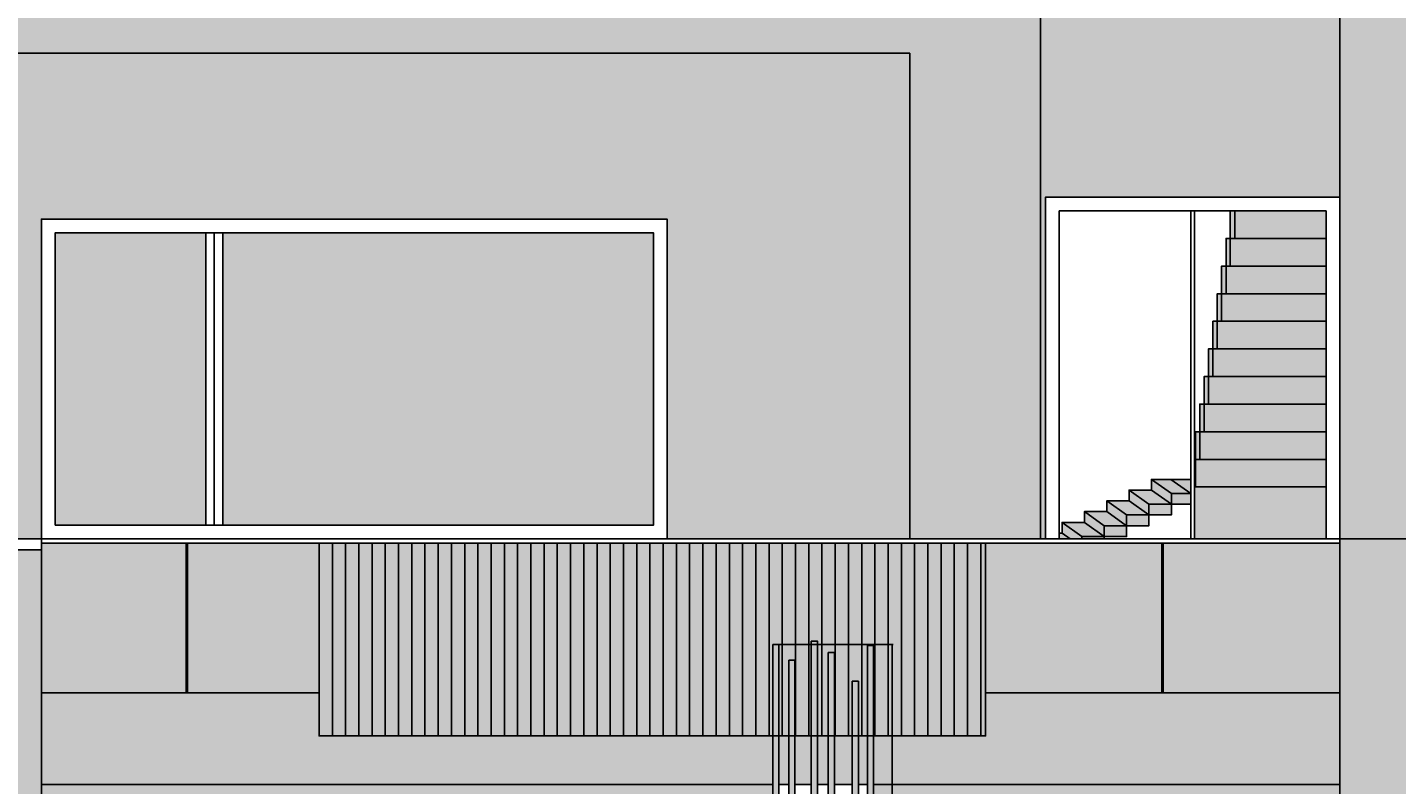
# Model space of a CAD drawing. Units: feet. Extents: x 2193 to 3502, y 890 to 1601.
# Tile 6 of 17: x 2466 to 2710, y 1225 to 1360. Entities that reach past the tile are written whole.
import ezdxf

# ---------------------------------------------------------------- set-up
doc = ezdxf.new("R2010")
doc.units = ezdxf.units.FT
for name, color, linetype, lineweight in [('A-ANNO-DIMS', 2, 'Continuous', 18), ('A-ELEV', 7, 'Continuous', 25), ('A-ELEV-PATT', 8, 'Continuous', 13)]:
    doc.layers.add(name, color=color, linetype=linetype, lineweight=lineweight)
doc.styles.get("Standard").update_dxf_attribs({"font": 'arial.ttf'})
doc.dimstyles.get("Standard").update_dxf_attribs({"dimtxt": 0.18, "dimasz": 0.18, "dimexe": 0.18, "dimexo": 0.0625, "dimgap": 0.09, "dimtad": 0, "dimtih": 1, "dimtoh": 1, "dimdec": 0, "dimzin": 0, "dimdsep": 46, "dimlunit": 3, "dimtxsty": 'Standard', "dimcen": 0.09, "dimadec": 0, "dimazin": 0, "dimtfac": 1, "dimtdec": 0, "dimtofl": 0, "dimtmove": 0, "dimatfit": 3, "dimfxl": 1, "dimtolj": 1, "dimtzin": 0, "dimarcsym": 0})

# ---------------------------------------------------------------- blocks, each defined once
blk = doc.blocks.new('STAIR-RAIL-A')
for p, q in [((6.38, 44.29), (6.38, 49.22)), ((5.61, 39.37), (5.61, 44.29)), ((5.61, 44.29), (6.38, 44.29)), ((23.45, 44.29), (6.38, 44.29)), ((6.38, 44.29), (6.38, 39.37)), ((4.83, 34.45), (4.83, 39.37)), ((4.83, 39.37), (5.61, 39.37)), ((23.45, 39.37), (5.61, 39.37)), ((5.61, 39.37), (5.61, 34.45)), ((4.05, 29.53), (4.05, 34.45)), ((4.05, 34.45), (4.83, 34.45)), ((23.45, 34.45), (4.83, 34.45)), ((4.83, 34.45), (4.83, 29.53)), ((3.27, 24.61), (3.27, 29.53)), ((3.27, 29.53), (4.05, 29.53)), ((23.45, 29.53), (4.05, 29.53)), ((4.05, 29.53), (4.05, 24.61)), ((2.49, 19.69), (2.49, 24.61)), ((2.49, 24.61), (3.27, 24.61)), ((23.45, 24.61), (3.27, 24.61)), ((3.27, 24.61), (3.27, 19.69)), ((1.71, 14.77), (1.71, 19.69)), ((1.71, 19.69), (2.49, 19.69)), ((23.45, 19.69), (2.49, 19.69)), ((2.49, 19.69), (2.49, 14.77)), ((0.93, 9.84), (0.93, 14.77)), ((0.93, 14.77), (1.71, 14.77)), ((23.45, 14.77), (1.71, 14.77)), ((1.71, 14.77), (1.71, 9.84)), ((0.16, 4.92), (0.16, 9.84)), ((0.16, 9.84), (0.93, 9.84)), ((23.45, 9.84), (0.93, 9.84)), ((0.93, 9.84), (0.93, 4.92)), ((23.45, 4.92), (0, 4.92)), ((23.45, 4.92), (0, 4.92)), ((0.16, 4.92), (0.16, 0)), ((23.45, 0), (0, 0)), ((23.45, 0), (0, 0))]:
    blk.add_line(p, q)
for points in [[(23.45, 44.29), (6.38, 44.29), (6.38, 49.22)], [(23.45, 39.37), (5.61, 39.37), (5.61, 44.29), (6.38, 44.29), (6.38, 39.37)], [(23.45, 34.45), (4.83, 34.45), (4.83, 39.37), (5.61, 39.37), (5.61, 34.45)], [(23.45, 29.53), (4.05, 29.53), (4.05, 34.45), (4.83, 34.45), (4.83, 29.53)], [(23.45, 24.61), (3.27, 24.61), (3.27, 29.53), (4.05, 29.53), (4.05, 24.61)], [(23.45, 19.69), (2.49, 19.69), (2.49, 24.61), (3.27, 24.61), (3.27, 19.69)], [(23.45, 14.77), (1.71, 14.77), (1.71, 19.69), (2.49, 19.69), (2.49, 14.77)], [(23.45, 9.84), (0.93, 9.84), (0.93, 14.77), (1.71, 14.77), (1.71, 9.84)], [(0.16, 0), (0.16, 4.92), (0.16, 9.84), (0.93, 9.84), (0.93, 4.92)]]:
    blk.add_lwpolyline(points)
blk = doc.blocks.new('METAL-FIN')
blk.add_lwpolyline([(0, 134.59), (1.1, 134.59), (1.1, 0), (0, 0)], close=True)
blk.add_lwpolyline([(0, 134.59), (1.1, 134.59), (1.1, 0), (0, 0)], close=True)
blk = doc.blocks.new('*D5')
at = {"layer": 'A-ANNO-DIMS', "color": 0, "lineweight": -2, "transparency": 16777216}
for p, q in [((2599.75, 1249.83), (2620.06, 1249.83)), ((2619.88, 1249.65), (2619.88, 1182.71)), ((2619.88, 1115.41), (2619.88, 1182.35)), ((2599.75, 1115.23), (2620.06, 1115.23))]:
    blk.add_line(p, q, dxfattribs=at)
at = {"layer": 'A-ANNO-DIMS', "color": 0, "transparency": 16777216}
for points in [[(2619.85, 1249.65), (2619.91, 1249.65), (2619.88, 1249.83)], [(2619.85, 1115.41), (2619.91, 1115.41), (2619.88, 1115.23)]]:
    blk.add_solid(points, dxfattribs=at)
at = {"layer": 'Defpoints', "color": 0, "transparency": 16777216}
for p in [(2599.69, 1249.83), (2619.88, 1249.83), (2599.69, 1115.23)]:
    blk.add_point(p, dxfattribs=at)
at = {"layer": 'A-ANNO-DIMS', "color": 0, "transparency": 16777216, "insert": (2619.88, 1182.53), "char_height": 0.18, "attachment_point": 5}
blk.add_mtext('\\A1;METAL FIN 135 TYP.', dxfattribs=at)
blk = doc.blocks.new('*D20')
at = {"layer": 'A-ANNO-DIMS', "color": 0, "lineweight": -2, "transparency": 16777216}
for p, q in [((2933.15, 1408.48), (2193.56, 1408.48)), ((2193.74, 1408.3), (2193.74, 1240.94)), ((2193.74, 1073.21), (2193.74, 1240.57)), ((2934.31, 1073.03), (2193.56, 1073.03))]:
    blk.add_line(p, q, dxfattribs=at)
at = {"layer": 'A-ANNO-DIMS', "color": 0, "transparency": 16777216}
for points in [[(2193.71, 1408.3), (2193.77, 1408.3), (2193.74, 1408.48)], [(2193.71, 1073.21), (2193.77, 1073.21), (2193.74, 1073.03)]]:
    blk.add_solid(points, dxfattribs=at)
at = {"layer": 'Defpoints', "color": 0, "transparency": 16777216}
for p in [(2193.74, 1408.48), (2933.21, 1408.48), (2934.37, 1073.03)]:
    blk.add_point(p, dxfattribs=at)
at = {"layer": 'A-ANNO-DIMS', "color": 0, "transparency": 16777216, "insert": (2193.74, 1240.76), "char_height": 0.18, "attachment_point": 5}
blk.add_mtext('\\A1;335.45', dxfattribs=at)
blk = doc.blocks.new('*D26')
at = {"layer": 'A-ANNO-DIMS', "color": 0, "lineweight": -2, "transparency": 16777216}
for p, q in [((2255.16, 950.89), (2255.16, 1601.47)), ((2255.34, 1601.29), (2507.42, 1601.29)), ((2760.29, 1601.29), (2508.21, 1601.29)), ((2760.47, 1541.11), (2760.47, 1601.47))]:
    blk.add_line(p, q, dxfattribs=at)
at = {"layer": 'A-ANNO-DIMS', "color": 0, "transparency": 16777216}
for points in [[(2255.34, 1601.32), (2255.34, 1601.26), (2255.16, 1601.29)], [(2760.29, 1601.32), (2760.29, 1601.26), (2760.47, 1601.29)]]:
    blk.add_solid(points, dxfattribs=at)
at = {"layer": 'Defpoints', "color": 0, "transparency": 16777216}
for p in [(2760.47, 1601.29), (2760.47, 1541.04), (2255.16, 950.82)]:
    blk.add_point(p, dxfattribs=at)
at = {"layer": 'A-ANNO-DIMS', "color": 0, "transparency": 16777216, "insert": (2507.82, 1601.29), "char_height": 0.18, "attachment_point": 5}
blk.add_mtext('\\A1;505.3', dxfattribs=at)
blk = doc.blocks.new('*D36')
at = {"layer": 'A-ANNO-DIMS', "color": 0, "lineweight": -2, "transparency": 16777216}
for p, q in [((2974.05, 1268.66), (2193.56, 1268.66)), ((2193.74, 1268.48), (2193.74, 1200.71)), ((2193.74, 1132.57), (2193.74, 1200.34)), ((2980.65, 1132.39), (2193.56, 1132.39))]:
    blk.add_line(p, q, dxfattribs=at)
at = {"layer": 'A-ANNO-DIMS', "color": 0, "transparency": 16777216}
for points in [[(2193.71, 1268.48), (2193.77, 1268.48), (2193.74, 1268.66)], [(2193.71, 1132.57), (2193.77, 1132.57), (2193.74, 1132.39)]]:
    blk.add_solid(points, dxfattribs=at)
at = {"layer": 'Defpoints', "color": 0, "transparency": 16777216}
for p in [(2193.74, 1268.66), (2974.12, 1268.66), (2980.72, 1132.39)]:
    blk.add_point(p, dxfattribs=at)
at = {"layer": 'A-ANNO-DIMS', "color": 0, "transparency": 16777216, "insert": (2193.74, 1200.53), "char_height": 0.18, "attachment_point": 5}
blk.add_mtext('\\A1;136.27', dxfattribs=at)
blk = doc.blocks.new('*D37')
at = {"layer": 'A-ANNO-DIMS', "color": 0, "lineweight": -2, "transparency": 16777216}
for p, q in [((2974.05, 1367.57), (2193.56, 1367.57)), ((2193.74, 1367.39), (2193.74, 1318.3)), ((2193.74, 1268.84), (2193.74, 1317.93)), ((2974.05, 1268.66), (2193.56, 1268.66))]:
    blk.add_line(p, q, dxfattribs=at)
at = {"layer": 'A-ANNO-DIMS', "color": 0, "transparency": 16777216}
for points in [[(2193.71, 1367.39), (2193.77, 1367.39), (2193.74, 1367.57)], [(2193.71, 1268.84), (2193.77, 1268.84), (2193.74, 1268.66)]]:
    blk.add_solid(points, dxfattribs=at)
at = {"layer": 'Defpoints', "color": 0, "transparency": 16777216}
for p in [(2193.74, 1367.57), (2974.12, 1367.57), (2974.12, 1268.66)]:
    blk.add_point(p, dxfattribs=at)
at = {"layer": 'A-ANNO-DIMS', "color": 0, "transparency": 16777216, "insert": (2193.74, 1318.12), "char_height": 0.18, "attachment_point": 5}
blk.add_mtext('\\A1;98.91', dxfattribs=at)

msp = doc.modelspace()

# ---------------------------------------------------------------- hatches: boundary and pattern name
at = {"layer": 'A-ELEV-PATT'}
h = msp.add_hatch(color=256, dxfattribs=at)
h.dxf.hatch_style = 1
h.paths.add_polyline_path([(2760.4733, 1541.0441), (2699.6322, 1541.0441), (2699.6322, 1512.3957), (2760.4733, 1512.3957)])
h.paths.add_polyline_path([(2760.4733, 1502.0763), (2699.6322, 1502.0763), (2699.6322, 1382.0763), (2760.4733, 1382.0763)])
h.paths.add_polyline_path([(2745.971, 1367.5739), (2699.6322, 1367.5739), (2699.6322, 1089.3627), (2760.4733, 1089.3627), (2760.4733, 1166.2327), (2745.971, 1166.2327)])
h.paths.add_polyline_path([(2754.7661, 1011.1246), (2690.9216, 1011.1246), (2690.9216, 993.3923), (2754.7661, 993.3923)])
h.paths.add_polyline_path([(2689.6008, 1011.1246), (2625.7563, 1011.1246), (2625.7563, 993.3923), (2689.6008, 993.3923)])
h.paths.add_polyline_path([(2599.6883, 1249.8256), (2598.591, 1249.8256), (2598.591, 1233.561), (2599.6883, 1233.561)])
h.paths.add_polyline_path([(2602.5204, 1247.0422), (2601.423, 1247.0422), (2601.423, 1233.561), (2602.5204, 1233.561)])
h.paths.add_polyline_path([(2606.5316, 1250.4403), (2605.4342, 1250.4403), (2605.4342, 1233.561), (2606.5316, 1233.561)])
h.paths.add_polyline_path([(2609.5836, 1248.4363), (2608.4862, 1248.4363), (2608.4862, 1233.561), (2609.5836, 1233.561)])
h.paths.add_polyline_path([(2613.8564, 1243.2956), (2612.759, 1243.2956), (2612.759, 1233.561), (2613.8564, 1233.561)])
h.paths.add_polyline_path([(2616.5596, 1249.6561), (2615.4622, 1249.6561), (2615.4622, 1233.561), (2616.5596, 1233.561)])
h.paths.add_polyline_path([(2599.6883, 1233.561), (2598.591, 1233.561), (2598.591, 1224.865), (2599.6883, 1224.865)])
h.paths.add_polyline_path([(2602.5204, 1233.561), (2601.423, 1233.561), (2601.423, 1224.865), (2602.5204, 1224.865)])
h.paths.add_polyline_path([(2606.5316, 1233.561), (2605.4342, 1233.561), (2605.4342, 1224.865), (2606.5316, 1224.865)])
h.paths.add_polyline_path([(2609.5836, 1233.561), (2608.4862, 1233.561), (2608.4862, 1224.865), (2609.5836, 1224.865)])
h.paths.add_polyline_path([(2613.8564, 1233.561), (2612.759, 1233.561), (2612.759, 1224.865), (2613.8564, 1224.865)])
h.paths.add_polyline_path([(2616.5596, 1233.561), (2615.4622, 1233.561), (2615.4622, 1224.865), (2616.5596, 1224.865)])
h.paths.add_polyline_path([(2599.6883, 1224.865), (2598.591, 1224.865), (2598.591, 1115.2331), (2599.6883, 1115.2331)])
h.paths.add_polyline_path([(2602.5204, 1224.865), (2601.423, 1224.865), (2601.423, 1112.4498), (2602.5204, 1112.4498)])
h.paths.add_polyline_path([(2606.5316, 1224.865), (2605.4342, 1224.865), (2605.4342, 1115.8479), (2606.5316, 1115.8479)])
h.paths.add_polyline_path([(2609.5836, 1224.865), (2608.4862, 1224.865), (2608.4862, 1113.8439), (2609.5836, 1113.8439)])
h.paths.add_polyline_path([(2616.5596, 1224.865), (2615.4622, 1224.865), (2615.4622, 1115.0637), (2616.5596, 1115.0637)])
h.paths.add_polyline_path([(2613.8564, 1224.865), (2612.759, 1224.865), (2612.759, 1108.7032), (2613.8564, 1108.7032)])
h = msp.add_hatch(color=256, dxfattribs=at)
h.dxf.hatch_style = 1
h.paths.add_polyline_path([(2760.4733, 1512.3957), (2586.1736, 1512.3957), (2586.1736, 1502.0763), (2602.8648, 1502.0763), (2699.5726, 1502.0763), (2699.6322, 1502.0763), (2760.4733, 1502.0763)])
h.paths.add_polyline_path([(2760.4733, 1382.0763), (2275.0482, 1382.0763), (2275.0482, 1367.5739), (2745.971, 1367.5739), (2745.971, 1166.2327), (2760.4733, 1166.2327)])
h.paths.add_polyline_path([(2468.2854, 1266.7092), (2294.8992, 1266.7092), (2294.8992, 1079.031), (2468.2854, 1079.031)])
h.paths.add_polyline_path([(2301.4984, 1260.11), (2461.6863, 1260.11), (2461.6863, 1085.6301), (2301.4984, 1085.6301)], flags=16)
h.paths.add_polyline_path([(2452.7821, 1241.1967), (2452.7821, 1217.2819), (2454.6216, 1217.2819), (2454.6216, 1133.1367), (2461.6863, 1133.1367), (2461.6863, 1132.3937), (2381.7172, 1132.3937), (2381.7172, 1085.6301), (2381.4675, 1085.6301), (2381.4675, 1132.3937), (2301.4984, 1132.3937), (2301.4984, 1133.1367), (2301.4984, 1217.2819), (2390.8933, 1217.2819), (2390.8933, 1241.1967)], flags=0)
h.paths.add_polyline_path([(2372.4936, 1214.8367), (2372.4936, 1133.1367), (2371.1246, 1133.1367), (2371.1246, 1214.8367), (2337.2323, 1214.8367), (2337.2323, 1133.1367), (2335.8632, 1133.1367), (2335.8632, 1214.8367), (2337.2323, 1214.8367)], flags=0)
h = msp.add_hatch(color=256, dxfattribs=at)
h.dxf.hatch_style = 1
h.paths.add_polyline_path([(2390.8933, 1367.5739), (2294.8992, 1367.5739), (2294.8992, 1329.5765), (2390.8933, 1329.5765)])
h.paths.add_polyline_path([(2489.6169, 1055.3069), (2585.8844, 1055.3069), (2585.8844, 1032.1935), (2620.0491, 1032.1935), (2620.0491, 1073.031), (2452.7821, 1073.031), (2452.7821, 1032.1935), (2489.6169, 1032.1935)])
h.paths.add_polyline_path([(2754.7661, 1073.031), (2654.2841, 1073.031), (2654.2841, 1047.0961), (2754.7661, 1047.0961)])
h.paths.add_polyline_path([(2643.9681, 1484.1152), (2699.5726, 1484.1152), (2699.5726, 1502.0763), (2602.8648, 1502.0763), (2602.8648, 1408.4814), (2643.9681, 1408.4814)])
h.paths.add_polyline_path([(2699.6322, 1367.5739), (2646.2844, 1367.5739), (2646.2844, 1268.6599), (2647.1841, 1268.6599), (2647.1841, 1329.5765), (2699.6322, 1329.5765)])
h.paths.add_polyline_path([(2699.6322, 1224.865), (2616.5596, 1224.865), (2616.5596, 1133.8558), (2647.1841, 1133.8558), (2647.1841, 1194.7724), (2699.6322, 1194.7724)])
h = msp.add_hatch(color=256, dxfattribs=at)
h.dxf.hatch_style = 1
h.paths.add_polyline_path([(2576.3428, 1407.7384), (2536.5416, 1407.7384), (2536.5416, 1406.15), (2536.5416, 1382.0763), (2576.3428, 1382.0763)])
h.paths.add_polyline_path([(2627.3548, 1407.7384), (2576.5924, 1407.7384), (2576.5924, 1382.0763), (2627.3548, 1382.0763)])
h.paths.add_polyline_path([(2667.9236, 1407.7384), (2627.6045, 1407.7384), (2627.6045, 1382.0763), (2667.9236, 1382.0763)])
h.paths.add_polyline_path([(2699.6322, 1407.7384), (2668.1733, 1407.7384), (2668.1733, 1382.0763), (2699.6322, 1382.0763)])
h.paths.add_polyline_path([(2497.5717, 1323.2248), (2470.7305, 1323.2248), (2470.7305, 1271.105), (2497.5717, 1271.105)])
h.paths.add_polyline_path([(2577.3219, 1323.2248), (2500.599, 1323.2248), (2500.599, 1271.105), (2577.3219, 1271.105)])
h.paths.add_polyline_path([(2388.4482, 1327.1314), (2343.4244, 1327.1314), (2343.4244, 1268.6599), (2388.4482, 1268.6599)])
h.paths.add_polyline_path([(2342.3682, 1327.1314), (2297.3443, 1327.1314), (2297.3443, 1268.6599), (2342.3682, 1268.6599)])
h.paths.add_polyline_path([(2335.8632, 1214.8367), (2301.4984, 1214.8367), (2301.4984, 1133.1367), (2335.8632, 1133.1367)])
h.paths.add_polyline_path([(2371.1246, 1214.8367), (2337.2323, 1214.8367), (2337.2323, 1133.1367), (2371.1246, 1133.1367)])
h.paths.add_polyline_path([(2390.8933, 1214.8367), (2372.4936, 1214.8367), (2372.4936, 1133.1367), (2390.8933, 1133.1367)])
h.paths.add_polyline_path([(2577.3219, 1188.4208), (2500.599, 1188.4208), (2500.599, 1136.3009), (2577.3219, 1136.3009)])
h.paths.add_polyline_path([(2497.5717, 1188.4208), (2470.7305, 1188.4208), (2470.7305, 1136.3009), (2497.5717, 1136.3009)])
h.paths.add_polyline_path([(2381.4675, 1132.3937), (2301.4984, 1132.3937), (2301.4984, 1085.6301), (2381.4675, 1085.6301)])
h.paths.add_polyline_path([(2461.6863, 1132.3937), (2381.7172, 1132.3937), (2381.7172, 1085.6301), (2461.6863, 1085.6301)])
h.paths.add_polyline_path([(2494.0463, 1133.1128), (2468.2854, 1133.1128), (2468.2854, 1089.3627), (2494.0463, 1089.3627)])
h.paths.add_polyline_path([(2517.7591, 1133.1128), (2494.296, 1133.1128), (2494.296, 1089.3627), (2517.7591, 1089.3627)])
h.paths.add_polyline_path([(2667.9236, 1133.1128), (2636.5184, 1133.1128), (2636.5184, 1089.3627), (2667.9236, 1089.3627)])
h.paths.add_polyline_path([(2699.6322, 1133.1128), (2668.1733, 1133.1128), (2668.1733, 1089.3627), (2699.6322, 1089.3627)])
h.paths.add_polyline_path([(2651.839, 1070.5859), (2638.7977, 1070.5859), (2638.7977, 1047.0961), (2651.839, 1047.0961)])
h.paths.add_polyline_path([(2637.6317, 1070.5859), (2625.7563, 1070.5859), (2625.7563, 1047.0961), (2637.6317, 1047.0961)])
h.paths.add_polyline_path([(2583.4393, 1052.8618), (2515.9216, 1052.8618), (2515.9216, 1032.1935), (2583.4393, 1032.1935)])
h.paths.add_polyline_path([(2514.4293, 1052.8618), (2492.062, 1052.8618), (2492.062, 1032.1935), (2514.4293, 1032.1935)])
h.paths.add_polyline_path([(2388.4482, 1038.8658), (2348.7682, 1038.8658), (2348.7682, 988.9597), (2388.4482, 988.9597)])
h.paths.add_polyline_path([(2346.3231, 1038.8658), (2309.0883, 1038.8658), (2309.0883, 988.9597), (2346.3231, 988.9597)])
h.paths.add_polyline_path([(2667.9236, 1267.9169), (2636.5184, 1267.9169), (2636.5184, 1241.1967), (2667.9236, 1241.1967)])
h.paths.add_polyline_path([(2699.6322, 1267.9169), (2668.1733, 1267.9169), (2668.1733, 1241.1967), (2699.6322, 1241.1967)])
h.paths.add_polyline_path([(2517.7591, 1267.9169), (2494.296, 1267.9169), (2494.296, 1241.1967), (2517.7591, 1241.1967)])
h.paths.add_polyline_path([(2494.0463, 1267.9169), (2468.2854, 1267.9169), (2468.2854, 1266.7092), (2468.2854, 1241.1967), (2494.0463, 1241.1967)])
h = msp.add_hatch(color=256, dxfattribs=at)
h.dxf.hatch_style = 1
h.paths.add_polyline_path([(2294.8992, 1367.5739), (2275.0482, 1367.5739), (2275.0482, 1382.0763), (2536.5416, 1382.0763), (2536.5416, 1406.15), (2256.3232, 1406.15), (2256.3232, 1089.3627), (2255.1574, 1089.3627), (2255.1574, 1073.031), (2294.8992, 1073.031)])
h.paths.add_polyline_path([(2517.7591, 1241.1967), (2468.2854, 1241.1967), (2468.2854, 1224.865), (2598.591, 1224.865), (2598.591, 1233.561), (2517.7591, 1233.561)])
h.paths.add_polyline_path([(2699.6322, 1241.1967), (2636.5184, 1241.1967), (2636.5184, 1233.561), (2616.5596, 1233.561), (2616.5596, 1224.865), (2699.6322, 1224.865)])
h.paths.add_polyline_path([(2615.4622, 1233.561), (2613.8564, 1233.561), (2613.8564, 1224.865), (2615.4622, 1224.865)])
h.paths.add_polyline_path([(2612.759, 1233.561), (2609.5836, 1233.561), (2609.5836, 1224.865), (2612.759, 1224.865)])
h.paths.add_polyline_path([(2608.4862, 1233.561), (2606.5316, 1233.561), (2606.5316, 1224.865), (2608.4862, 1224.865)])
h.paths.add_polyline_path([(2605.4342, 1233.561), (2602.5204, 1233.561), (2602.5204, 1224.865), (2605.4342, 1224.865)])
h.paths.add_polyline_path([(2601.423, 1233.561), (2599.6883, 1233.561), (2599.6883, 1224.865), (2601.423, 1224.865)])
h.paths.add_polyline_path([(2517.7591, 1089.3627), (2468.2854, 1089.3627), (2468.2854, 1079.031), (2294.8992, 1079.031), (2294.8992, 1073.031), (2390.8933, 1073.031), (2452.7821, 1073.031), (2760.4733, 1073.031), (2760.4733, 1089.3627), (2699.6322, 1089.3627), (2636.5184, 1089.3627), (2636.5184, 1081.7269), (2517.7591, 1081.7269)])
h = msp.add_hatch(color=256, dxfattribs=at)
h.dxf.hatch_style = 1
h.paths.add_polyline_path([(2452.7821, 1355.2199), (2622.9814, 1355.2199), (2622.9814, 1268.6599), (2646.2844, 1268.6599), (2646.2844, 1367.5739), (2390.8933, 1367.5739), (2390.8933, 1268.6599), (2452.7821, 1268.6599)])
h.paths.add_polyline_path([(2452.7821, 1016.4), (2431.9134, 1016.4), (2431.9134, 1032.1935), (2452.7821, 1032.1935), (2452.7821, 1073.031), (2390.8933, 1073.031), (2390.8933, 956.8829), (2452.7821, 956.8829)])
h.paths.add_polyline_path([(2452.7821, 1241.1967), (2390.8933, 1241.1967), (2390.8933, 1133.1367), (2452.7821, 1133.1367)])
h.paths.add_polyline_path([(2636.5184, 1267.9169), (2517.7591, 1267.9169), (2517.7591, 1233.561), (2598.591, 1233.561), (2598.591, 1249.8256), (2599.6883, 1249.8256), (2599.6883, 1233.561), (2601.423, 1233.561), (2601.423, 1247.0422), (2602.5204, 1247.0422), (2602.5204, 1233.561), (2605.4342, 1233.561), (2605.4342, 1250.4403), (2606.5316, 1250.4403), (2606.5316, 1233.561), (2608.4862, 1233.561), (2608.4862, 1248.4363), (2609.5836, 1248.4363), (2609.5836, 1233.561), (2612.759, 1233.561), (2612.759, 1243.2956), (2613.8564, 1243.2956), (2613.8564, 1233.561), (2615.4622, 1233.561), (2615.4622, 1249.6561), (2616.5596, 1249.6561), (2616.5596, 1233.561), (2636.5184, 1233.561)])
h.paths.add_polyline_path([(2601.423, 1133.1128), (2599.6883, 1133.1128), (2599.6883, 1115.2331), (2598.591, 1115.2331), (2598.591, 1133.1128), (2517.7591, 1133.1128), (2517.7591, 1081.7269), (2636.5184, 1081.7269), (2636.5184, 1133.1128), (2616.5596, 1133.1128), (2616.5596, 1115.0637), (2615.4622, 1115.0637), (2615.4622, 1133.1128), (2613.8564, 1133.1128), (2613.8564, 1108.7032), (2612.759, 1108.7032), (2612.759, 1133.1128), (2609.5836, 1133.1128), (2609.5836, 1113.8439), (2608.4862, 1113.8439), (2608.4862, 1133.1128), (2606.5316, 1133.1128), (2606.5316, 1115.8479), (2605.4342, 1115.8479), (2605.4342, 1133.1128), (2602.5204, 1133.1128), (2602.5204, 1112.4498), (2601.423, 1112.4498)])
h = msp.add_hatch(color=256, dxfattribs=at)
h.dxf.hatch_style = 1
h.paths.add_polyline_path([(2622.9814, 1355.2199), (2452.7821, 1355.2199), (2452.7821, 1268.6599), (2468.2854, 1268.6599), (2468.2854, 1325.6699), (2579.767, 1325.6699), (2579.767, 1268.6599), (2622.9814, 1268.6599)])
h.paths.add_polyline_path([(2598.591, 1224.865), (2468.2854, 1224.865), (2468.2854, 1190.8659), (2579.767, 1190.8659), (2579.767, 1133.8558), (2598.591, 1133.8558)])
h.paths.add_polyline_path([(2390.8933, 1241.1967), (2301.4984, 1241.1967), (2301.4984, 1224.865), (2390.8933, 1224.865)])
h.paths.add_polyline_path([(3070.1101, 1073.031), (2940.0814, 1073.031), (2940.0814, 956.5285), (2940.6598, 956.8829), (3070.1101, 956.8829), (3070.1101, 986.5146), (2985.8599, 986.5146), (2985.8599, 1041.3109), (3070.1101, 1041.3109)])
h = msp.add_hatch(color=256, dxfattribs=at)
h.dxf.hatch_style = 1
h.paths.add_polyline_path([(2697.1871, 1322.2098), (2680.1178, 1322.2098), (2680.1178, 1317.2882), (2697.1871, 1317.2882)])
h.paths.add_polyline_path([(2697.1871, 1327.1314), (2680.8966, 1327.1314), (2680.8966, 1322.2098), (2697.1871, 1322.2098)])
h.paths.add_polyline_path([(2697.1871, 1317.2882), (2679.3391, 1317.2882), (2679.3391, 1312.3666), (2697.1871, 1312.3666)])
h.paths.add_polyline_path([(2697.1871, 1312.3666), (2678.5604, 1312.3666), (2678.5604, 1307.445), (2697.1871, 1307.445)])
h.paths.add_polyline_path([(2697.1871, 1307.445), (2677.7817, 1307.445), (2677.7817, 1302.5234), (2697.1871, 1302.5234)])
h.paths.add_polyline_path([(2697.1871, 1302.5234), (2677.0029, 1302.5234), (2677.0029, 1297.6018), (2697.1871, 1297.6018)])
h.paths.add_polyline_path([(2697.1871, 1297.6018), (2676.2242, 1297.6018), (2676.2242, 1292.6802), (2697.1871, 1292.6802)])
h.paths.add_polyline_path([(2697.1871, 1292.6802), (2675.4455, 1292.6802), (2675.4455, 1287.7586), (2697.1871, 1287.7586)])
h.paths.add_polyline_path([(2697.1871, 1287.7586), (2674.6667, 1287.7586), (2673.888, 1287.7586), (2673.888, 1282.8371), (2673.888, 1277.9155), (2673.7332, 1268.6599), (2697.1871, 1268.6599)])
h.paths.add_polyline_path([(2662.0707, 1275.4405), (2658.0881, 1275.4405), (2661.6386, 1272.9217), (2665.6211, 1272.9217)])
h.paths.add_polyline_path([(2666.0533, 1279.2756), (2666.0533, 1277.358), (2669.6037, 1274.8393), (2669.6037, 1276.7569)])
h.paths.add_polyline_path([(2669.5328, 1279.2756), (2666.0533, 1279.2756), (2669.6037, 1276.7569), (2673.0832, 1276.7569)])
h.paths.add_polyline_path([(2673.0832, 1279.2756), (2669.5328, 1279.2756), (2673.0832, 1276.7569)], flags=17)
h.paths.add_polyline_path([(2673.0832, 1276.7569), (2669.6037, 1276.7569), (2669.6037, 1274.8393), (2673.0832, 1274.8393)])
h.paths.add_polyline_path([(2669.6037, 1274.8393), (2665.6211, 1274.8393), (2665.6211, 1272.9217), (2669.6037, 1272.9217)])
h.paths.add_polyline_path([(2666.0533, 1277.358), (2662.0707, 1277.358), (2665.6211, 1274.8393), (2669.6037, 1274.8393)])
h.paths.add_polyline_path([(2662.0707, 1277.358), (2662.0707, 1275.4405), (2665.6211, 1272.9217), (2665.6211, 1274.8393)])
h.paths.add_polyline_path([(2665.6211, 1272.9217), (2661.6386, 1272.9217), (2661.6386, 1271.0041), (2665.6211, 1271.0041)])
h.paths.add_polyline_path([(2658.0881, 1275.4405), (2658.0881, 1273.5229), (2661.6386, 1271.0041), (2661.6386, 1272.9217)])
h.paths.add_polyline_path([(2661.6386, 1271.0041), (2657.656, 1271.0041), (2657.656, 1269.0866), (2661.6386, 1269.0866)])
h.paths.add_polyline_path([(2658.0881, 1273.5229), (2654.1056, 1273.5229), (2657.656, 1271.0041), (2661.6386, 1271.0041)])
h.paths.add_polyline_path([(2654.1056, 1273.5229), (2654.1056, 1271.6053), (2657.656, 1269.0866), (2657.656, 1271.0041)])
h.paths.add_polyline_path([(2650.123, 1271.6053), (2650.123, 1269.6877), (2651.5719, 1268.6599), (2653.6734, 1268.6599), (2653.6734, 1269.0866)])
h.paths.add_polyline_path([(2654.1056, 1271.6053), (2650.123, 1271.6053), (2653.6734, 1269.0866), (2657.656, 1269.0866)])
h.paths.add_polyline_path([(2650.123, 1269.6877), (2649.6293, 1269.6877), (2649.6293, 1268.6599), (2651.5719, 1268.6599)])
h.paths.add_polyline_path([(2657.656, 1269.0866), (2653.6734, 1269.0866), (2653.6734, 1268.6599), (2657.656, 1268.6599)])
h.paths.add_polyline_path([(2697.1871, 1192.3273), (2680.8966, 1192.3273), (2680.8966, 1187.4057), (2697.1871, 1187.4057)])
h.paths.add_polyline_path([(2697.1871, 1187.4057), (2680.1178, 1187.4057), (2680.1178, 1182.4841), (2697.1871, 1182.4841)])
h.paths.add_polyline_path([(2697.1871, 1177.5625), (2678.5604, 1177.5625), (2678.5604, 1172.641), (2697.1871, 1172.641)])
h.paths.add_polyline_path([(2697.1871, 1182.4841), (2679.3391, 1182.4841), (2679.3391, 1177.5625), (2697.1871, 1177.5625)])
h.paths.add_polyline_path([(2697.1871, 1172.641), (2677.7817, 1172.641), (2677.7817, 1167.7194), (2697.1871, 1167.7194)])
h.paths.add_polyline_path([(2697.1871, 1167.7194), (2677.0029, 1167.7194), (2677.0029, 1162.7978), (2697.1871, 1162.7978)])
h.paths.add_polyline_path([(2697.1871, 1162.7978), (2676.2242, 1162.7978), (2676.2242, 1157.8762), (2697.1871, 1157.8762)])
h.paths.add_polyline_path([(2697.1871, 1143.1114), (2673.7332, 1143.1114), (2673.7332, 1133.8558), (2697.1871, 1133.8558)])
h.paths.add_polyline_path([(2697.1871, 1148.033), (2673.888, 1148.033), (2673.888, 1143.1114), (2697.1871, 1143.1114)])
h.paths.add_polyline_path([(2697.1871, 1152.9546), (2674.6667, 1152.9546), (2674.6667, 1148.033), (2697.1871, 1148.033)])
h.paths.add_polyline_path([(2697.1871, 1157.8762), (2675.4455, 1157.8762), (2675.4455, 1152.9546), (2697.1871, 1152.9546)])
h.paths.add_polyline_path([(2673.0832, 1141.9528), (2669.6037, 1141.9528), (2669.6037, 1140.0352), (2673.0832, 1140.0352)])
h.paths.add_polyline_path([(2669.5328, 1144.4716), (2666.0533, 1144.4716), (2669.6037, 1141.9528), (2673.0832, 1141.9528)])
h.paths.add_polyline_path([(2673.0832, 1144.4716), (2669.5328, 1144.4716), (2673.0832, 1141.9528)], flags=17)
h.paths.add_polyline_path([(2666.0533, 1142.554), (2662.0707, 1142.554), (2665.6211, 1140.0352), (2669.6037, 1140.0352)])
h.paths.add_polyline_path([(2666.0533, 1144.4716), (2666.0533, 1142.554), (2669.6037, 1140.0352), (2669.6037, 1141.9528)])
h.paths.add_polyline_path([(2669.6037, 1140.0352), (2665.6211, 1140.0352), (2665.6211, 1138.1177), (2669.6037, 1138.1177)])
h.paths.add_polyline_path([(2665.6211, 1140.0352), (2662.0707, 1142.554), (2662.0707, 1140.6364), (2665.6211, 1138.1177)])
h.paths.add_polyline_path([(2653.6734, 1134.2825), (2650.123, 1136.8013), (2650.123, 1134.8837), (2651.5719, 1133.8558), (2653.6734, 1133.8558)])
h.paths.add_polyline_path([(2654.1056, 1136.8013), (2650.123, 1136.8013), (2653.6734, 1134.2825), (2657.656, 1134.2825)])
h.paths.add_polyline_path([(2657.656, 1134.2825), (2653.6734, 1134.2825), (2653.6734, 1133.8558), (2657.656, 1133.8558)])
h.paths.add_polyline_path([(2661.6386, 1136.2001), (2657.656, 1136.2001), (2657.656, 1134.2825), (2661.6386, 1134.2825)])
h.paths.add_polyline_path([(2657.656, 1136.2001), (2654.1056, 1138.7188), (2654.1056, 1136.8013), (2657.656, 1134.2825)])
h.paths.add_polyline_path([(2658.0881, 1138.7188), (2654.1056, 1138.7188), (2657.656, 1136.2001), (2661.6386, 1136.2001)])
h.paths.add_polyline_path([(2658.0881, 1140.6364), (2658.0881, 1138.7188), (2661.6386, 1136.2001), (2661.6386, 1138.1177)])
h.paths.add_polyline_path([(2662.0707, 1140.6364), (2658.0881, 1140.6364), (2661.6386, 1138.1177), (2665.6211, 1138.1177)])
h.paths.add_polyline_path([(2665.6211, 1138.1177), (2661.6386, 1138.1177), (2661.6386, 1136.2001), (2665.6211, 1136.2001)])
h.paths.add_polyline_path([(2650.123, 1134.8837), (2649.6293, 1134.8837), (2649.6293, 1133.8558), (2651.5719, 1133.8558)])
h = msp.add_hatch(color=256, dxfattribs=at)
h.dxf.hatch_style = 1
h.paths.add_polyline_path([(2680.8966, 1327.1314), (2680.1178, 1327.1314), (2680.1178, 1322.2098), (2680.8966, 1322.2098)])
h.paths.add_polyline_path([(2680.1178, 1322.2098), (2679.3391, 1322.2098), (2679.3391, 1317.2882), (2680.1178, 1317.2882)])
h.paths.add_polyline_path([(2679.3391, 1317.2882), (2678.5604, 1317.2882), (2678.5604, 1312.3666), (2679.3391, 1312.3666)])
h.paths.add_polyline_path([(2678.5604, 1312.3666), (2677.7817, 1312.3666), (2677.7817, 1307.445), (2678.5604, 1307.445)])
h.paths.add_polyline_path([(2677.7817, 1307.445), (2677.0029, 1307.445), (2677.0029, 1302.5234), (2677.7817, 1302.5234)])
h.paths.add_polyline_path([(2677.0029, 1302.5234), (2676.2242, 1302.5234), (2676.2242, 1297.6018), (2677.0029, 1297.6018)])
h.paths.add_polyline_path([(2676.2242, 1297.6018), (2675.4455, 1297.6018), (2675.4455, 1292.6802), (2676.2242, 1292.6802)])
h.paths.add_polyline_path([(2675.4455, 1292.6802), (2674.6667, 1292.6802), (2674.6667, 1287.7586), (2675.4455, 1287.7586)])
h.paths.add_polyline_path([(2680.8966, 1192.3273), (2680.1178, 1192.3273), (2680.1178, 1187.4057), (2680.8966, 1187.4057)])
h.paths.add_polyline_path([(2680.1178, 1187.4057), (2679.3391, 1187.4057), (2679.3391, 1182.4841), (2680.1178, 1182.4841)])
h.paths.add_polyline_path([(2679.3391, 1182.4841), (2678.5604, 1182.4841), (2678.5604, 1177.5625), (2679.3391, 1177.5625)])
h.paths.add_polyline_path([(2678.5604, 1177.5625), (2677.7817, 1177.5625), (2677.7817, 1172.641), (2678.5604, 1172.641)])
h.paths.add_polyline_path([(2677.7817, 1172.641), (2677.0029, 1172.641), (2677.0029, 1167.7194), (2677.7817, 1167.7194)])

# ---------------------------------------------------------------- linework, layer by layer
at = {"layer": 'A-ELEV'}
for p, q in [((2452.7821, 1355.2199), (2622.9814, 1355.2199)), ((2680.8966, 1327.1314), (2680.8966, 1322.2098)), ((2680.8966, 1327.1314), (2680.8966, 1322.2098)), ((2669.6037, 1276.7569), (2666.0533, 1279.2756)), ((2666.0533, 1279.2756), (2669.5328, 1279.2756)), ((2666.0533, 1277.358), (2666.0533, 1279.2756)), ((2669.5328, 1279.2756), (2673.0832, 1276.7569)), ((2669.5328, 1279.2756), (2673.0832, 1279.2756)), ((2662.0707, 1277.358), (2666.0533, 1277.358)), ((2662.0707, 1275.4405), (2662.0707, 1277.358)), ((2662.0707, 1277.358), (2666.0533, 1277.358)), ((2665.6211, 1274.8393), (2662.0707, 1277.358)), ((2666.0533, 1277.358), (2669.6037, 1274.8393)), ((2669.6037, 1274.8393), (2669.6037, 1276.7569)), ((2669.6037, 1276.7569), (2673.0832, 1276.7569)), ((2654.1056, 1271.6053), (2654.1056, 1273.5229)), ((2654.1056, 1271.6053), (2654.1056, 1273.5229)), ((2654.1056, 1273.5229), (2658.0881, 1273.5229)), ((2654.1056, 1273.5229), (2657.656, 1271.0041)), ((2658.0881, 1273.5229), (2658.0881, 1275.4405)), ((2658.0881, 1273.5229), (2658.0881, 1275.4405)), ((2658.0881, 1275.4405), (2662.0707, 1275.4405)), ((2658.0881, 1275.4405), (2661.6386, 1272.9217)), ((2658.0881, 1273.5229), (2661.6386, 1271.0041)), ((2662.0707, 1275.4405), (2665.6211, 1272.9217)), ((2665.6211, 1272.9217), (2665.6211, 1274.8393)), ((2665.6211, 1274.8393), (2669.6037, 1274.8393)), ((2669.6037, 1274.8393), (2673.0832, 1274.8393)), ((2669.6037, 1272.9217), (2669.6037, 1274.8393)), ((2650.123, 1269.6877), (2650.123, 1271.6053)), ((2650.123, 1269.6877), (2650.123, 1271.6053)), ((2650.123, 1271.6053), (2654.1056, 1271.6053)), ((2650.123, 1271.6053), (2653.6734, 1269.0866)), ((2654.1056, 1271.6053), (2657.656, 1269.0866)), ((2661.6386, 1271.0041), (2661.6386, 1272.9217)), ((2661.6386, 1272.9217), (2665.6211, 1272.9217)), ((2665.6211, 1271.0041), (2665.6211, 1272.9217)), ((2665.6211, 1272.9217), (2669.6037, 1272.9217)), ((2649.6293, 1269.6877), (2650.123, 1269.6877)), ((2650.123, 1269.6877), (2651.5719, 1268.6599)), ((2653.6734, 1268.6599), (2653.6734, 1269.0866)), ((2653.6734, 1268.6599), (2653.6734, 1269.0866)), ((2653.6734, 1269.0866), (2657.656, 1269.0866)), ((2657.656, 1269.0866), (2657.656, 1271.0041)), ((2657.656, 1271.0041), (2661.6386, 1271.0041)), ((2657.656, 1268.6599), (2657.656, 1269.0866)), ((2657.656, 1269.0866), (2661.6386, 1269.0866)), ((2661.6386, 1269.0866), (2661.6386, 1271.0041)), ((2661.6386, 1271.0041), (2665.6211, 1271.0041)), ((2468.2854, 1241.1967), (2517.7591, 1241.1967)), ((2468.2854, 1241.1967), (2517.7591, 1241.1967)), ((2636.5184, 1241.1967), (2699.6322, 1241.1967)), ((2636.5184, 1241.1967), (2699.6322, 1241.1967)), ((2468.2854, 1224.865), (2598.591, 1224.865)), ((2599.6883, 1224.865), (2601.423, 1224.865)), ((2602.5204, 1224.865), (2605.4342, 1224.865)), ((2606.5316, 1224.865), (2608.4862, 1224.865)), ((2609.5836, 1224.865), (2612.759, 1224.865)), ((2613.8564, 1224.865), (2615.4622, 1224.865)), ((2616.5596, 1224.865), (2699.6322, 1224.865))]:
    msp.add_line(p, q, dxfattribs=at)
for points in [[(2760.4733, 1415.3157), (2760.4733, 1089.3627), (2699.6322, 1089.3627), (2699.6322, 1367.5739)], [(2760.4733, 1415.3157), (2760.4733, 1089.3627), (2699.6322, 1089.3627), (2699.6322, 1367.5739)], [(2622.9814, 1367.5739), (2646.2844, 1367.5739), (2646.2844, 1268.6599), (2622.9814, 1268.6599), (2622.9814, 1355.2199), (2452.7821, 1355.2199), (2452.7821, 1266.7092), (2390.8933, 1266.7092), (2390.8933, 1367.5739)], [(2622.9814, 1367.5739), (2646.2844, 1367.5739), (2646.2844, 1268.6599), (2622.9814, 1268.6599), (2622.9814, 1355.2199)], [(2649.6293, 1268.6599), (2649.6293, 1327.1314), (2697.1871, 1327.1314), (2697.1871, 1268.6599)], [(2649.6293, 1268.6599), (2649.6293, 1327.1314), (2697.1871, 1327.1314), (2697.1871, 1268.6599)], [(2669.5328, 1279.2756), (2666.0533, 1279.2756), (2666.0533, 1277.358), (2669.6037, 1274.8393), (2669.6037, 1276.7569)], [(2666.0533, 1279.2756), (2669.6037, 1276.7569), (2673.0832, 1276.7569), (2669.5328, 1279.2756), (2673.0832, 1279.2756)], [(2669.6037, 1274.8393), (2665.6211, 1274.8393), (2662.0707, 1277.358), (2662.0707, 1275.4405), (2665.6211, 1272.9217), (2665.6211, 1274.8393)], [(2661.6386, 1272.9217), (2661.6386, 1271.0041), (2658.0881, 1273.5229), (2654.1056, 1273.5229), (2657.656, 1271.0041), (2661.6386, 1271.0041)], [(2657.656, 1268.6599), (2657.656, 1269.0866), (2661.6386, 1269.0866), (2661.6386, 1271.0041), (2665.6211, 1271.0041), (2665.6211, 1272.9217), (2669.6037, 1272.9217), (2669.6037, 1274.8393), (2673.0832, 1274.8393)], [(2662.0707, 1275.4405), (2658.0881, 1275.4405), (2661.6386, 1272.9217), (2665.6211, 1272.9217)], [(2657.656, 1271.0041), (2657.656, 1269.0866), (2654.1056, 1271.6053), (2650.123, 1271.6053), (2653.6734, 1269.0866), (2657.656, 1269.0866)], [(2699.6322, 1267.9169), (2468.2854, 1267.9169), (2468.2854, 1268.6599), (2699.6322, 1268.6599)], [(2699.6322, 1267.9169), (2468.2854, 1267.9169), (2468.2854, 1268.6599), (2699.6322, 1268.6599)], [(2649.6293, 1269.6877), (2650.123, 1269.6877), (2651.5719, 1268.6599)], [(2494.296, 1267.9169), (2494.296, 1241.1967), (2494.0463, 1241.1967), (2494.0463, 1267.9169)], [(2494.296, 1267.9169), (2494.296, 1241.1967), (2494.0463, 1241.1967), (2494.0463, 1267.9169)], [(2636.5184, 1267.9169), (2636.5184, 1233.561), (2517.7591, 1233.561), (2517.7591, 1267.9169)], [(2598.591, 1233.561), (2517.7591, 1233.561), (2517.7591, 1267.9169)], [(2520.1169, 1267.9169), (2520.1169, 1233.561), (2518.938, 1233.561)], [(2522.4747, 1267.9169), (2522.4747, 1233.561), (2521.2958, 1233.561)], [(2524.8326, 1267.9169), (2524.8326, 1233.561), (2523.6536, 1233.561)], [(2527.1904, 1267.9169), (2527.1904, 1233.561), (2526.0115, 1233.561)], [(2529.5482, 1267.9169), (2529.5482, 1233.561), (2528.3693, 1233.561)], [(2531.9061, 1267.9169), (2531.9061, 1233.561), (2530.7272, 1233.561)], [(2534.2639, 1267.9169), (2534.2639, 1233.561), (2533.085, 1233.561)], [(2536.6217, 1267.9169), (2536.6217, 1233.561), (2535.4428, 1233.561)], [(2538.9796, 1267.9169), (2538.9796, 1233.561), (2537.8007, 1233.561)], [(2541.3374, 1267.9169), (2541.3374, 1233.561), (2540.1585, 1233.561)], [(2543.6953, 1267.9169), (2543.6953, 1233.561), (2542.5163, 1233.561)], [(2546.0531, 1267.9169), (2546.0531, 1233.561), (2544.8742, 1233.561)], [(2548.4109, 1267.9169), (2548.4109, 1233.561), (2547.232, 1233.561)], [(2550.7688, 1267.9169), (2550.7688, 1233.561), (2549.5899, 1233.561)], [(2553.1266, 1267.9169), (2553.1266, 1233.561), (2551.9477, 1233.561)], [(2555.4844, 1267.9169), (2555.4844, 1233.561), (2554.3055, 1233.561)], [(2557.8423, 1267.9169), (2557.8423, 1233.561), (2556.6634, 1233.561)], [(2560.2001, 1267.9169), (2560.2001, 1233.561), (2559.0212, 1233.561)], [(2562.558, 1267.9169), (2562.558, 1233.561), (2561.379, 1233.561)], [(2564.9158, 1267.9169), (2564.9158, 1233.561), (2563.7369, 1233.561)], [(2567.2736, 1267.9169), (2567.2736, 1233.561), (2566.0947, 1233.561)], [(2569.6315, 1267.9169), (2569.6315, 1233.561), (2568.4525, 1233.561)], [(2571.9893, 1267.9169), (2571.9893, 1233.561), (2570.8104, 1233.561)], [(2574.3471, 1267.9169), (2574.3471, 1233.561), (2573.1682, 1233.561)], [(2576.705, 1267.9169), (2576.705, 1233.561), (2575.5261, 1233.561)], [(2579.0628, 1267.9169), (2579.0628, 1233.561), (2577.8839, 1233.561)], [(2581.4207, 1267.9169), (2581.4207, 1233.561), (2580.2417, 1233.561)], [(2583.7785, 1267.9169), (2583.7785, 1233.561), (2582.5996, 1233.561)], [(2586.1363, 1267.9169), (2586.1363, 1233.561), (2584.9574, 1233.561)], [(2588.4942, 1267.9169), (2588.4942, 1233.561), (2587.3152, 1233.561)], [(2590.852, 1267.9169), (2590.852, 1233.561), (2589.6731, 1233.561)], [(2593.2098, 1267.9169), (2593.2098, 1233.561), (2592.0309, 1233.561)], [(2595.5677, 1267.9169), (2595.5677, 1233.561), (2594.3888, 1233.561)], [(2597.9255, 1267.9169), (2597.9255, 1233.561), (2596.7466, 1233.561)], [(2600.2833, 1267.9169), (2600.2833, 1233.561), (2599.6883, 1233.561)], [(2602.6412, 1267.9169), (2602.6412, 1233.561), (2602.5204, 1233.561)], [(2604.999, 1267.9169), (2604.999, 1233.561), (2603.8201, 1233.561)], [(2607.3569, 1267.9169), (2607.3569, 1233.561), (2606.5316, 1233.561)], [(2609.7147, 1267.9169), (2609.7147, 1233.561), (2609.5836, 1233.561)], [(2612.0725, 1267.9169), (2612.0725, 1233.561), (2610.8936, 1233.561)], [(2614.4304, 1267.9169), (2614.4304, 1233.561), (2613.8564, 1233.561)], [(2636.5184, 1267.9169), (2636.5184, 1233.561), (2616.5596, 1233.561)], [(2616.7882, 1267.9169), (2616.7882, 1233.561), (2616.5596, 1233.561)], [(2619.146, 1267.9169), (2619.146, 1233.561), (2617.9671, 1233.561)], [(2621.5039, 1267.9169), (2621.5039, 1233.561), (2620.325, 1233.561)], [(2623.8617, 1267.9169), (2623.8617, 1233.561), (2622.6828, 1233.561)], [(2626.2196, 1267.9169), (2626.2196, 1233.561), (2625.0406, 1233.561)], [(2628.5774, 1267.9169), (2628.5774, 1233.561), (2627.3985, 1233.561)], [(2630.9352, 1267.9169), (2630.9352, 1233.561), (2629.7563, 1233.561)], [(2633.2931, 1267.9169), (2633.2931, 1233.561), (2632.1141, 1233.561)], [(2635.6509, 1267.9169), (2635.6509, 1233.561), (2634.472, 1233.561)], [(2668.1733, 1267.9169), (2668.1733, 1241.1967), (2667.9236, 1241.1967), (2667.9236, 1267.9169)], [(2668.1733, 1267.9169), (2668.1733, 1241.1967), (2667.9236, 1241.1967), (2667.9236, 1267.9169)], [(2601.423, 1233.561), (2599.6883, 1233.561)], [(2605.4342, 1233.561), (2602.5204, 1233.561)], [(2608.4862, 1233.561), (2606.5316, 1233.561)], [(2612.759, 1233.561), (2609.5836, 1233.561)], [(2615.4622, 1233.561), (2613.8564, 1233.561)]]:
    msp.add_lwpolyline(points, dxfattribs=at)
for points in [[(2699.6322, 1268.6599), (2647.1841, 1268.6599), (2647.1841, 1329.5765), (2699.6322, 1329.5765)], [(2699.6322, 1268.6599), (2647.1841, 1268.6599), (2647.1841, 1329.5765), (2699.6322, 1329.5765)], [(2468.2854, 1268.6599), (2579.767, 1268.6599), (2579.767, 1325.6699), (2468.2854, 1325.6699)], [(2468.2854, 1268.6599), (2579.767, 1268.6599), (2579.767, 1325.6699), (2468.2854, 1325.6699)], [(2673.0832, 1327.1314), (2673.7332, 1327.1314), (2673.7332, 1268.6599), (2673.0832, 1268.6599)], [(2673.0832, 1327.1314), (2673.7332, 1327.1314), (2673.7332, 1268.6599), (2673.0832, 1268.6599)], [(2470.7305, 1271.105), (2577.3219, 1271.105), (2577.3219, 1323.2248), (2470.7305, 1323.2248)], [(2470.7305, 1271.105), (2577.3219, 1271.105), (2577.3219, 1323.2248), (2470.7305, 1323.2248)], [(2497.5717, 1323.2248), (2499.0853, 1323.2248), (2499.0853, 1271.105), (2497.5717, 1271.105)], [(2497.5717, 1323.2248), (2499.0853, 1323.2248), (2499.0853, 1271.105), (2497.5717, 1271.105)], [(2499.0853, 1323.2248), (2500.599, 1323.2248), (2500.599, 1271.105), (2499.0853, 1271.105)], [(2499.0853, 1323.2248), (2500.599, 1323.2248), (2500.599, 1271.105), (2499.0853, 1271.105)], [(2294.8992, 1266.7092), (2468.2854, 1266.7092), (2468.2854, 1268.6599), (2294.8992, 1268.6599)], [(2294.8992, 1266.7092), (2468.2854, 1266.7092), (2468.2854, 1268.6599), (2294.8992, 1268.6599)], [(2294.8992, 1079.031), (2468.2854, 1079.031), (2468.2854, 1266.7092), (2294.8992, 1266.7092)], [(2294.8992, 1079.031), (2468.2854, 1079.031), (2468.2854, 1266.7092), (2294.8992, 1266.7092)]]:
    msp.add_lwpolyline(points, close=True, dxfattribs=at)

# ---------------------------------------------------------------- block references
for name, p in [('STAIR-RAIL-A', (2673.733, 1277.9151)), ('METAL-FIN', (2598.591, 1115.233)), ('METAL-FIN', (2605.4342, 1115.8477)), ('METAL-FIN', (2615.4622, 1115.0636)), ('METAL-FIN', (2601.423, 1112.4497)), ('METAL-FIN', (2608.4862, 1113.8437)), ('METAL-FIN', (2612.759, 1108.7031))]:
    msp.add_blockref(name, p, dxfattribs=at)

# ---------------------------------------------------------------- dimensions: what is measured, and where the dimension line sits
at = {"layer": 'A-ANNO-DIMS'}
dim = msp.add_linear_dim(base=(2760.4733, 1601.2941), p1=(2255.1574, 950.8228), p2=(2760.4733, 1541.0441), dimstyle='Standard', override={"dimdec": 1, "dimlfac": 1, "dimrnd": 0, "dimzin": 0, "dimdsep": 46, "dimlunit": 2}, dxfattribs=at)
dim.commit()
dim.dimension.update_dxf_attribs({"geometry": '*D26', "text_midpoint": (2507.8154, 1601.2941)})
for base, p1, p2, picture, middle in [((2193.7417, 1408.4814), (2934.3742, 1073.031), (2933.2085, 1408.4814), '*D20', (2193.7417, 1240.7562)), ((2193.7417, 1367.5739), (2974.116, 1268.6599), (2974.116, 1367.5739), '*D37', (2193.7417, 1318.1169)), ((2193.7417, 1268.6599), (2980.7151, 1132.3937), (2974.116, 1268.6599), '*D36', (2193.7417, 1200.5268))]:
    dim = msp.add_linear_dim(base=base, p1=p1, p2=p2, angle=90, dimstyle='Standard', override={"dimdec": 2, "dimlfac": 1, "dimrnd": 0, "dimzin": 0, "dimdsep": 46, "dimlunit": 2}, dxfattribs=at)
    dim.commit()
    dim.dimension.update_dxf_attribs({"geometry": picture, "text_midpoint": middle})
dim = msp.add_linear_dim(base=(2619.8772, 1249.8256), p1=(2599.6883, 1115.2331), p2=(2599.6883, 1249.8256), angle=90, text='METAL FIN <> TYP.', dimstyle='Standard', override={"dimdec": 0, "dimlfac": 1, "dimrnd": 0, "dimzin": 0, "dimdsep": 46, "dimlunit": 2}, dxfattribs=at)
dim.commit()
dim.dimension.update_dxf_attribs({"geometry": '*D5', "text_midpoint": (2619.8772, 1182.5293)})

doc.saveas('drawing.dxf')
